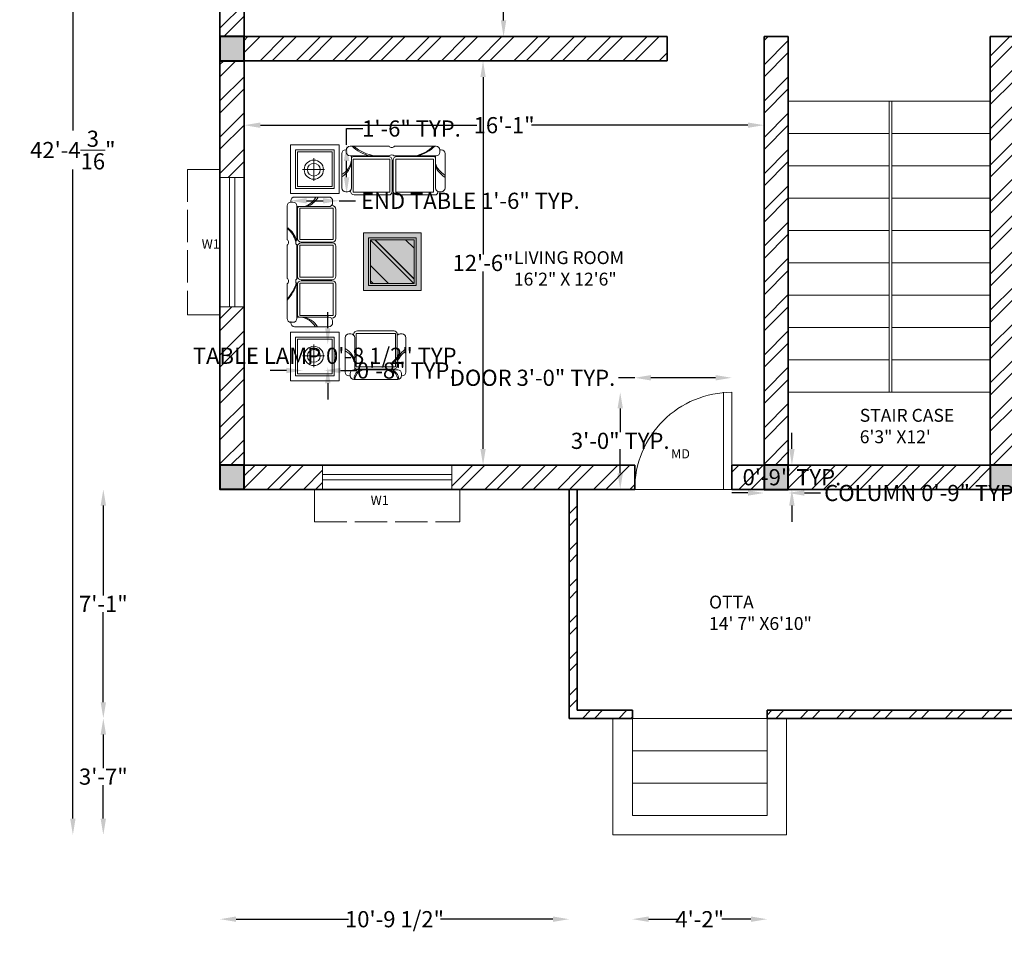
# Model space of a CAD drawing. Units: inches. Extents: x 3614 to 4242, y 2406 to 3033.
# Tile 1 of 10: x 3614 to 3980, y 2406 to 2749. Entities that reach past the tile are written whole.
import ezdxf

# ---------------------------------------------------------------- set-up
doc = ezdxf.new("R2010")
doc.units = ezdxf.units.IN
doc.linetypes.add('ACAD_ISO02W100', pattern=[15, 12, -3])
for name, color, linetype, lineweight in [('A-ANNO-DIMS', 2, 'Continuous', 18), ('A-ANNO-TEXT', 7, 'Continuous', 18), ('A-AREA-IDEN', 7, 'Continuous', 25), ('A-COLS', 7, 'Continuous', 40), ('A-COLS-PATT', 252, 'Continuous', 18), ('A-DOOR', 3, 'Continuous', 18), ('A-FLOR-STRS', 7, 'Continuous', 18), ('A-FURN', 8, 'Continuous', 18), ('A-FURN-PATT', 252, 'Continuous', 13), ('A-GLAZ', 4, 'Continuous', 18), ('A-GLAZ-OVHD', 8, 'ACAD_ISO02W100', 13), ('A-WALL', 7, 'Continuous', 35), ('A-WALL-PATT', 252, 'Continuous', 13)]:
    doc.layers.add(name, color=color, linetype=linetype, lineweight=lineweight)
doc.styles.get("Standard").update_dxf_attribs({"font": 'arial.ttf'})
doc.dimstyles.get("Standard").update_dxf_attribs({"dimtxt": 6, "dimasz": 6, "dimexe": 0.18, "dimexo": 0.0625, "dimgap": 0.09, "dimtad": 0, "dimtih": 1, "dimtoh": 1, "dimdec": 4, "dimzin": 0, "dimdsep": 46, "dimlunit": 4, "dimtxsty": 'Standard', "dimcen": 0.09, "dimse1": 1, "dimse2": 1, "dimadec": 0, "dimazin": 0, "dimtfac": 1, "dimtdec": 4, "dimtofl": 0, "dimtmove": 0, "dimatfit": 3, "dimfxl": 1, "dimtolj": 1, "dimtzin": 0, "dimarcsym": 0})

# ---------------------------------------------------------------- blocks, each defined once
blk = doc.blocks.new('*D15')
at = {"layer": 'A-ANNO-DIMS', "color": 0, "lineweight": -2, "transparency": 16777216}
for p, q in [((3793.63, 2939.34), (3793.63, 2846.99)), ((3793.63, 2748.34), (3793.63, 2840.69))]:
    blk.add_line(p, q, dxfattribs=at)
at = {"layer": 'A-ANNO-DIMS', "color": 0, "transparency": 16777216}
for points in [[(3792.63, 2939.34), (3794.63, 2939.34), (3793.63, 2945.34)], [(3792.63, 2748.34), (3794.63, 2748.34), (3793.63, 2742.34)]]:
    blk.add_solid(points, dxfattribs=at)
at = {"layer": 'Defpoints', "color": 0, "transparency": 16777216}
for p in [(3799.84, 2945.34), (3793.63, 2742.34), (3799.84, 2742.34)]:
    blk.add_point(p, dxfattribs=at)
at = {"layer": 'A-ANNO-DIMS', "color": 0, "transparency": 16777216, "insert": (3793.63, 2843.84), "char_height": 6, "attachment_point": 5}
blk.add_mtext('\\A1;16\'-11"', dxfattribs=at)
blk = doc.blocks.new('*D17')
at = {"layer": 'A-ANNO-DIMS', "color": 0, "lineweight": -2, "transparency": 16777216}
for p, q in [((3786.02, 2727.34), (3786.02, 2661.49)), ((3786.02, 2589.34), (3786.02, 2655.19))]:
    blk.add_line(p, q, dxfattribs=at)
at = {"layer": 'A-ANNO-DIMS', "color": 0, "transparency": 16777216}
for points in [[(3785.02, 2727.34), (3787.02, 2727.34), (3786.02, 2733.34)], [(3785.02, 2589.34), (3787.02, 2589.34), (3786.02, 2583.34)]]:
    blk.add_solid(points, dxfattribs=at)
at = {"layer": 'Defpoints', "color": 0, "transparency": 16777216}
for p in [(3831.84, 2733.34), (3786.02, 2583.34), (3830.34, 2583.34)]:
    blk.add_point(p, dxfattribs=at)
at = {"layer": 'A-ANNO-DIMS', "color": 0, "transparency": 16777216, "insert": (3786.02, 2658.34), "char_height": 6, "attachment_point": 5}
blk.add_mtext('\\A1;12\'-6"', dxfattribs=at)
blk = doc.blocks.new('*D18')
at = {"layer": 'A-ANNO-DIMS', "color": 0, "lineweight": -2, "transparency": 16777216}
for p, q in [((3703.34, 2709.47), (3783.72, 2709.47)), ((3884.34, 2709.47), (3803.95, 2709.47))]:
    blk.add_line(p, q, dxfattribs=at)
at = {"layer": 'A-ANNO-DIMS', "color": 0, "transparency": 16777216}
for points in [[(3703.34, 2710.47), (3703.34, 2708.47), (3697.34, 2709.47)], [(3884.34, 2710.47), (3884.34, 2708.47), (3890.34, 2709.47)]]:
    blk.add_solid(points, dxfattribs=at)
at = {"layer": 'Defpoints', "color": 0, "transparency": 16777216}
for p in [(3890.34, 2709.47), (3697.34, 2600.55), (3890.34, 2600.55)]:
    blk.add_point(p, dxfattribs=at)
at = {"layer": 'A-ANNO-DIMS', "color": 0, "transparency": 16777216, "insert": (3793.84, 2709.47), "char_height": 6, "attachment_point": 5}
blk.add_mtext('\\A1;16\'-1"', dxfattribs=at)
blk = doc.blocks.new('*D26')
at = {"layer": 'A-ANNO-DIMS', "color": 0, "lineweight": -2, "transparency": 16777216}
for p, q in [((3633.72, 2948.34), (3633.72, 2707.46)), ((3633.72, 2452.14), (3633.72, 2693.02))]:
    blk.add_line(p, q, dxfattribs=at)
at = {"layer": 'A-ANNO-DIMS', "color": 0, "transparency": 16777216}
for points in [[(3632.72, 2948.34), (3634.72, 2948.34), (3633.72, 2954.34)], [(3632.72, 2452.14), (3634.72, 2452.14), (3633.72, 2446.14)]]:
    blk.add_solid(points, dxfattribs=at)
at = {"layer": 'Defpoints', "color": 0, "transparency": 16777216}
for p in [(3688.34, 2954.34), (3633.72, 2446.14), (3688.34, 2446.14)]:
    blk.add_point(p, dxfattribs=at)
at = {"layer": 'A-ANNO-DIMS', "color": 0, "transparency": 16777216, "insert": (3633.72, 2700.24), "char_height": 6, "attachment_point": 5}
blk.add_mtext('\\A1;42\'-4{\\H1x;\\S3/16;}"', dxfattribs=at)
blk = doc.blocks.new('WINDOW-W1-48IN')
for p, q in [((48, 9), (0, 9)), ((0, 9), (0, 0)), ((48, 0), (48, 9)), ((0, 5.5), (48, 5.5)), ((0, 3.5), (48, 3.5)), ((0, 0), (48, 0))]:
    blk.add_line(p, q)
blk = doc.blocks.new('SHADE-W1')
for p, q in [((0, 0), (0, 12)), ((0, 12), (51, 12)), ((51, 12), (54, 12)), ((54, 12), (54, 0)), ((3, 0), (0, 0))]:
    blk.add_line(p, q)
blk = doc.blocks.new('COLUMN-9X9')
blk.add_lwpolyline([(9, 9), (0, 9), (0, 0), (9, 0)], close=True)
blk = doc.blocks.new('DOOR-SWING-36IN')
for p, q in [((0, 36), (0, 0)), ((0, 0), (0, 36)), ((3, 0), (3, 36))]:
    blk.add_line(p, q)
blk.add_arc((0, 36), 36, 270, 0)
blk = doc.blocks.new('TABLE-END-SQUARE')
for p, q in [((18.1, 18.1), (0, 18.1)), ((0, 18.1), (0, 0)), ((16.2, 16.2), (1.91, 16.2)), ((1.91, 16.2), (1.91, 1.91)), ((15.48, 15.48), (2.62, 15.48)), ((2.62, 15.48), (2.62, 2.62)), ((15.48, 2.62), (15.48, 15.48)), ((16.2, 1.91), (16.2, 16.2)), ((18.1, 0), (18.1, 18.1)), ((0, 0), (18.1, 0)), ((1.91, 1.91), (16.2, 1.91)), ((2.62, 2.62), (15.48, 2.62))]:
    blk.add_line(p, q)
blk = doc.blocks.new('LAMP-TABLE-PLAN')
for p, q in [((4.15, 0), (4.15, 8.41)), ((0, 4.15), (8.06, 4.15))]:
    blk.add_line(p, q)
for radius in [3.57, 2.38]:
    blk.add_circle((4.15, 4.15), radius)
blk = doc.blocks.new('*D39')
at = {"layer": 'A-ANNO-DIMS', "color": 0, "lineweight": -2, "transparency": 16777216}
for p, q in [((3884.34, 2572.99), (3878.34, 2572.99)), ((3905.34, 2572.99), (3911.34, 2572.99))]:
    blk.add_line(p, q, dxfattribs=at)
at = {"layer": 'A-ANNO-DIMS', "color": 0, "transparency": 16777216}
for points in [[(3884.34, 2573.99), (3884.34, 2571.99), (3890.34, 2572.99)], [(3905.34, 2573.99), (3905.34, 2571.99), (3899.34, 2572.99)]]:
    blk.add_solid(points, dxfattribs=at)
at = {"layer": 'Defpoints', "color": 0, "transparency": 16777216}
for p in [(3890.34, 2574.34), (3899.34, 2574.34), (3899.34, 2572.99)]:
    blk.add_point(p, dxfattribs=at)
at = {"layer": 'A-ANNO-DIMS', "color": 0, "transparency": 16777216, "insert": (3949, 2572.99), "char_height": 6, "attachment_point": 5}
blk.add_mtext('\\A1;COLUMN 0\'-9" TYP.', dxfattribs=at)
blk = doc.blocks.new('*D40')
at = {"layer": 'A-ANNO-DIMS', "color": 0, "lineweight": -2, "transparency": 16777216}
for p, q in [((3900.69, 2589.34), (3900.69, 2595.34)), ((3900.69, 2568.34), (3900.69, 2562.34))]:
    blk.add_line(p, q, dxfattribs=at)
at = {"layer": 'A-ANNO-DIMS', "color": 0, "transparency": 16777216}
for points in [[(3899.69, 2589.34), (3901.69, 2589.34), (3900.69, 2583.34)], [(3899.69, 2568.34), (3901.69, 2568.34), (3900.69, 2574.34)]]:
    blk.add_solid(points, dxfattribs=at)
at = {"layer": 'Defpoints', "color": 0, "transparency": 16777216}
for p in [(3899.34, 2583.34), (3900.69, 2583.34), (3899.34, 2574.34)]:
    blk.add_point(p, dxfattribs=at)
at = {"layer": 'A-ANNO-DIMS', "color": 0, "transparency": 16777216, "insert": (3900.69, 2578.84), "char_height": 6, "attachment_point": 5}
blk.add_mtext('\\A1;0\'-9" TYP.', dxfattribs=at)
blk = doc.blocks.new('*D49')
at = {"layer": 'A-ANNO-DIMS', "color": 0, "lineweight": -2, "transparency": 16777216}
for p, q in [((3842.34, 2615.74), (3836.34, 2615.74)), ((3872.34, 2615.74), (3848.34, 2615.74))]:
    blk.add_line(p, q, dxfattribs=at)
at = {"layer": 'A-ANNO-DIMS', "color": 0, "transparency": 16777216}
for points in [[(3848.34, 2616.74), (3848.34, 2614.74), (3842.34, 2615.74)], [(3872.34, 2616.74), (3872.34, 2614.74), (3878.34, 2615.74)]]:
    blk.add_solid(points, dxfattribs=at)
at = {"layer": 'Defpoints', "color": 0, "transparency": 16777216}
for p in [(3842.34, 2615.74), (3842.34, 2610.34), (3878.34, 2610.34)]:
    blk.add_point(p, dxfattribs=at)
at = {"layer": 'A-ANNO-DIMS', "color": 0, "transparency": 16777216, "insert": (3804.37, 2615.74), "char_height": 6, "attachment_point": 5}
blk.add_mtext('\\A1;DOOR 3\'-0" TYP.', dxfattribs=at)
blk = doc.blocks.new('*D50')
at = {"layer": 'A-ANNO-DIMS', "color": 0, "lineweight": -2, "transparency": 16777216}
for p, q in [((3836.94, 2604.34), (3836.94, 2595.5)), ((3836.94, 2580.34), (3836.94, 2589.19))]:
    blk.add_line(p, q, dxfattribs=at)
at = {"layer": 'A-ANNO-DIMS', "color": 0, "transparency": 16777216}
for points in [[(3835.94, 2604.34), (3837.94, 2604.34), (3836.94, 2610.34)], [(3835.94, 2580.34), (3837.94, 2580.34), (3836.94, 2574.34)]]:
    blk.add_solid(points, dxfattribs=at)
at = {"layer": 'Defpoints', "color": 0, "transparency": 16777216}
for p in [(3842.34, 2610.34), (3836.94, 2574.34), (3842.34, 2574.34)]:
    blk.add_point(p, dxfattribs=at)
at = {"layer": 'A-ANNO-DIMS', "color": 0, "transparency": 16777216, "insert": (3836.94, 2592.34), "char_height": 6, "attachment_point": 5}
blk.add_mtext('\\A1;3\'-0" TYP.', dxfattribs=at)
blk = doc.blocks.new('*D59')
at = {"layer": 'A-ANNO-DIMS', "color": 0, "lineweight": -2, "transparency": 16777216}
for p, q in [((3720.53, 2681.41), (3726.63, 2681.41)), ((3732.63, 2681.41), (3738.63, 2681.41))]:
    blk.add_line(p, q, dxfattribs=at)
at = {"layer": 'A-ANNO-DIMS', "color": 0, "transparency": 16777216}
for points in [[(3720.53, 2682.41), (3720.53, 2680.41), (3714.53, 2681.41)], [(3726.63, 2682.41), (3726.63, 2680.41), (3732.63, 2681.41)]]:
    blk.add_solid(points, dxfattribs=at)
at = {"layer": 'Defpoints', "color": 0, "transparency": 16777216}
for p in [(3714.53, 2684.13), (3732.63, 2684.13), (3732.63, 2681.41)]:
    blk.add_point(p, dxfattribs=at)
at = {"layer": 'A-ANNO-DIMS', "color": 0, "transparency": 16777216, "insert": (3781.31, 2681.41), "char_height": 6, "attachment_point": 5}
blk.add_mtext('\\A1;END TABLE 1\'-6" TYP.', dxfattribs=at)
blk = doc.blocks.new('*D60')
at = {"layer": 'A-ANNO-DIMS', "color": 0, "lineweight": -2, "transparency": 16777216}
for p, q in [((3735.35, 2702.23), (3735.35, 2708.23)), ((3735.35, 2708.23), (3741.35, 2708.23)), ((3735.35, 2690.13), (3735.35, 2696.23))]:
    blk.add_line(p, q, dxfattribs=at)
at = {"layer": 'A-ANNO-DIMS', "color": 0, "transparency": 16777216}
for points in [[(3734.35, 2696.23), (3736.35, 2696.23), (3735.35, 2702.23)], [(3734.35, 2690.13), (3736.35, 2690.13), (3735.35, 2684.13)]]:
    blk.add_solid(points, dxfattribs=at)
at = {"layer": 'Defpoints', "color": 0, "transparency": 16777216}
for p in [(3732.63, 2702.23), (3735.35, 2702.23), (3732.63, 2684.13)]:
    blk.add_point(p, dxfattribs=at)
at = {"layer": 'A-ANNO-DIMS', "color": 0, "transparency": 16777216, "insert": (3759.44, 2708.23), "char_height": 6, "attachment_point": 5}
blk.add_mtext('\\A1;1\'-6" TYP.', dxfattribs=at)
blk = doc.blocks.new('*D61')
at = {"layer": 'A-ANNO-DIMS', "color": 0, "lineweight": -2, "transparency": 16777216}
for p, q in [((3728.37, 2634.11), (3728.37, 2640.11)), ((3728.37, 2613.7), (3728.37, 2607.7))]:
    blk.add_line(p, q, dxfattribs=at)
at = {"layer": 'A-ANNO-DIMS', "color": 0, "transparency": 16777216}
for points in [[(3727.37, 2634.11), (3729.37, 2634.11), (3728.37, 2628.11)], [(3727.37, 2613.7), (3729.37, 2613.7), (3728.37, 2619.7)]]:
    blk.add_solid(points, dxfattribs=at)
at = {"layer": 'Defpoints', "color": 0, "transparency": 16777216}
for p in [(3727.11, 2628.11), (3728.37, 2628.11), (3727.11, 2619.7)]:
    blk.add_point(p, dxfattribs=at)
at = {"layer": 'A-ANNO-DIMS', "color": 0, "transparency": 16777216, "insert": (3728.37, 2623.9), "char_height": 6, "attachment_point": 5}
blk.add_mtext('\\A1;TABLE LAMP 0\'-8 1/2" TYP.', dxfattribs=at)
blk = doc.blocks.new('*D62')
at = {"layer": 'A-ANNO-DIMS', "color": 0, "lineweight": -2, "transparency": 16777216}
for p, q in [((3713.04, 2618.44), (3707.04, 2618.44)), ((3733.11, 2618.44), (3739.11, 2618.44))]:
    blk.add_line(p, q, dxfattribs=at)
at = {"layer": 'A-ANNO-DIMS', "color": 0, "transparency": 16777216}
for points in [[(3713.04, 2619.44), (3713.04, 2617.44), (3719.04, 2618.44)], [(3733.11, 2619.44), (3733.11, 2617.44), (3727.11, 2618.44)]]:
    blk.add_solid(points, dxfattribs=at)
at = {"layer": 'Defpoints', "color": 0, "transparency": 16777216}
for p in [(3719.04, 2619.7), (3727.11, 2619.7), (3727.11, 2618.44)]:
    blk.add_point(p, dxfattribs=at)
at = {"layer": 'A-ANNO-DIMS', "color": 0, "transparency": 16777216, "insert": (3757.48, 2618.44), "char_height": 6, "attachment_point": 5}
blk.add_mtext('\\A1;0\'-8" TYP.', dxfattribs=at)
blk = doc.blocks.new('*D67')
at = {"layer": 'A-ANNO-DIMS', "color": 0, "lineweight": -2, "transparency": 16777216}
for p, q in [((3694.34, 2414.84), (3736.04, 2414.84)), ((3811.95, 2414.84), (3770.25, 2414.84))]:
    blk.add_line(p, q, dxfattribs=at)
at = {"layer": 'A-ANNO-DIMS', "color": 0, "transparency": 16777216}
for points in [[(3694.34, 2415.84), (3694.34, 2413.84), (3688.34, 2414.84)], [(3811.95, 2415.84), (3811.95, 2413.84), (3817.95, 2414.84)]]:
    blk.add_solid(points, dxfattribs=at)
at = {"layer": 'Defpoints', "color": 0, "transparency": 16777216}
for p in [(3688.34, 2574.34), (3817.95, 2574.34), (3817.95, 2414.84)]:
    blk.add_point(p, dxfattribs=at)
at = {"layer": 'A-ANNO-DIMS', "color": 0, "transparency": 16777216, "insert": (3753.14, 2414.84), "char_height": 6, "attachment_point": 5}
blk.add_mtext('\\A1;10\'-9 1/2"', dxfattribs=at)
blk = doc.blocks.new('*D68')
at = {"layer": 'A-ANNO-DIMS', "color": 0, "lineweight": -2, "transparency": 16777216}
for p, q in [((3645.04, 2568.34), (3645.04, 2534.94)), ((3645.04, 2495.34), (3645.04, 2528.74))]:
    blk.add_line(p, q, dxfattribs=at)
at = {"layer": 'A-ANNO-DIMS', "color": 0, "transparency": 16777216}
for points in [[(3644.04, 2568.34), (3646.04, 2568.34), (3645.04, 2574.34)], [(3644.04, 2495.34), (3646.04, 2495.34), (3645.04, 2489.34)]]:
    blk.add_solid(points, dxfattribs=at)
at = {"layer": 'Defpoints', "color": 0, "transparency": 16777216}
for p in [(3645.04, 2574.34), (3817.95, 2574.34), (3817.95, 2489.34)]:
    blk.add_point(p, dxfattribs=at)
at = {"layer": 'A-ANNO-DIMS', "color": 0, "transparency": 16777216, "insert": (3645.04, 2531.84), "char_height": 6, "attachment_point": 5}
blk.add_mtext('\\A1;7\'-1"', dxfattribs=at)
blk = doc.blocks.new('*D69')
at = {"layer": 'A-ANNO-DIMS', "color": 0, "lineweight": -2, "transparency": 16777216}
for p, q in [((3847.46, 2414.84), (3858.28, 2414.84)), ((3885.48, 2414.84), (3874.65, 2414.84))]:
    blk.add_line(p, q, dxfattribs=at)
at = {"layer": 'A-ANNO-DIMS', "color": 0, "transparency": 16777216}
for points in [[(3847.46, 2415.84), (3847.46, 2413.84), (3841.46, 2414.84)], [(3885.48, 2415.84), (3885.48, 2413.84), (3891.48, 2414.84)]]:
    blk.add_solid(points, dxfattribs=at)
at = {"layer": 'Defpoints', "color": 0, "transparency": 16777216}
for p in [(3841.46, 2453.34), (3891.48, 2453.34), (3891.48, 2414.84)]:
    blk.add_point(p, dxfattribs=at)
at = {"layer": 'A-ANNO-DIMS', "color": 0, "transparency": 16777216, "insert": (3866.47, 2414.84), "char_height": 6, "attachment_point": 5}
blk.add_mtext('\\A1;4\'-2"', dxfattribs=at)
blk = doc.blocks.new('*D70')
at = {"layer": 'A-ANNO-DIMS', "color": 0, "lineweight": -2, "transparency": 16777216}
for p, q in [((3645.04, 2483.34), (3645.04, 2470.9)), ((3645.04, 2452.14), (3645.04, 2464.59))]:
    blk.add_line(p, q, dxfattribs=at)
at = {"layer": 'A-ANNO-DIMS', "color": 0, "transparency": 16777216}
for points in [[(3644.04, 2483.34), (3646.04, 2483.34), (3645.04, 2489.34)], [(3644.04, 2452.14), (3646.04, 2452.14), (3645.04, 2446.14)]]:
    blk.add_solid(points, dxfattribs=at)
at = {"layer": 'Defpoints', "color": 0, "transparency": 16777216}
for p in [(3645.04, 2489.34), (3834.26, 2489.34), (3834.26, 2446.14)]:
    blk.add_point(p, dxfattribs=at)
at = {"layer": 'A-ANNO-DIMS', "color": 0, "transparency": 16777216, "insert": (3645.04, 2467.74), "char_height": 6, "attachment_point": 5}
blk.add_mtext('\\A1;3\'-7"', dxfattribs=at)

msp = doc.modelspace()

# ---------------------------------------------------------------- hatches: boundary and pattern name
at = {"layer": 'A-COLS-PATT'}
h = msp.add_hatch(color=256, dxfattribs=at)
h.dxf.hatch_style = 1
h.paths.add_polyline_path([(3697.336, 2954.34049), (3688.336, 2954.34049), (3688.336, 2945.34049), (3697.336, 2945.34049)])
h.paths.add_polyline_path([(3818.336, 2954.34049), (3809.336, 2954.34049), (3809.336, 2945.34049), (3818.336, 2945.34049)])
h.paths.add_polyline_path([(3818.336, 2787.28572), (3809.336, 2787.28572), (3809.336, 2778.34049), (3818.336, 2778.34049)])
h.paths.add_polyline_path([(3697.336, 2742.34049), (3688.336, 2742.34049), (3688.336, 2733.34049), (3697.336, 2733.34049)])
h.paths.add_polyline_path([(3697.336, 2583.37355), (3688.336, 2583.37355), (3688.336, 2574.37355), (3697.336, 2574.37355)])
h.paths.add_polyline_path([(3899.336, 2583.34049), (3890.336, 2583.34049), (3890.336, 2574.34049), (3899.336, 2574.34049)])
h.paths.add_polyline_path([(3983.336, 2583.34049), (3974.336, 2583.34049), (3974.336, 2574.34049), (3983.336, 2574.34049)])
h.paths.add_polyline_path([(4153.336, 2583.34049), (4144.336, 2583.34049), (4144.336, 2574.34049), (4153.336, 2574.34049)])
h.paths.add_polyline_path([(4153.336, 2742.34049), (4144.336, 2742.34049), (4144.336, 2733.34049), (4153.336, 2733.34049)])
h.paths.add_polyline_path([(4153.336, 2795.34049), (4144.336, 2795.34049), (4144.336, 2786.34049), (4153.336, 2786.34049)])
h.paths.add_polyline_path([(3983.336, 2795.31105), (3974.336, 2795.31105), (3974.336, 2786.34049), (3983.336, 2786.34049)])
h.paths.add_polyline_path([(4153.336, 2954.34049), (4144.36882, 2954.34049), (4144.36882, 2945.34049), (4153.336, 2945.34049)])
h.paths.add_polyline_path([(3982.96188, 2954.34049), (3973.96188, 2954.34049), (3973.96188, 2945.34049), (3982.96188, 2945.34049)])
at = {"layer": 'A-FURN-PATT'}
h = msp.add_hatch(dxfattribs=at)
h.set_pattern_fill('CROSS', color=256, scale=0.833737, angle=135, style=0)
h.set_pattern_definition([(135, (1285.79775, 1101.19767), (-0.294770579, 0), [0.104217138, -0.312651413]), (225, (1285.79775, 1101.27136), (0, -0.294770579), [0.104217138, -0.312651413])])
h.paths.add_polyline_path([(3763.05675, 2669.55465), (3741.6178, 2669.55465), (3741.6178, 2648.11569), (3763.05675, 2648.11569)])
h = msp.add_hatch(dxfattribs=at)
h.set_pattern_fill('AR-RROOF', color=256, scale=11.91053, angle=135, style=0)
h.set_pattern_definition([(135, (1285.798, 1101.198), (-26.950453, 10.10642), [178.65795, -23.82106, 59.55265, -11.91053]), (135, (1270.385, 1108.188), (-2.779265, -19.6233), [35.7316, -3.93047, 71.46318, -8.9329]), (135, (1274.428, 1098.25), (-49.437237, 38.151735), [95.28424, -16.67474, 47.64212, -11.91053])])
h.paths.add_polyline_path([(3760.43644, 2666.93433), (3744.23811, 2666.93433), (3744.23811, 2650.73601), (3760.43644, 2650.73601)])
at = {"layer": 'A-WALL-PATT'}
h = msp.add_hatch(dxfattribs=at)
h.set_pattern_fill('ANSI32', color=256)
h.paths.add_polyline_path([(4153.336, 2945.34049), (4144.336, 2945.34049), (4144.336, 2902.95478), (4153.336, 2902.95478)])
h.paths.add_polyline_path([(4144.36882, 2954.34049), (4089.01458, 2954.34049), (4089.01458, 2945.34049), (4144.36882, 2945.34049)])
h.paths.add_polyline_path([(3818.336, 2945.34049), (3809.336, 2945.34049), (3809.336, 2787.28572), (3818.336, 2787.28572)])
h.paths.add_polyline_path([(3697.336, 2846.73438), (3688.336, 2846.73438), (3688.336, 2742.34049), (3697.336, 2742.34049)])
h.paths.add_polyline_path([(3854.336, 2742.34049), (3853.36389, 2742.34049), (3818.336, 2742.34049), (3809.336, 2742.34049), (3697.336, 2742.34049), (3697.336, 2733.34049), (3809.336, 2733.34049), (3854.336, 2733.34049)])
h.paths.add_polyline_path([(3697.336, 2733.34049), (3688.336, 2733.34049), (3688.336, 2690.05693), (3697.336, 2690.05693)])
h.paths.add_polyline_path([(3697.336, 2642.05693), (3688.336, 2642.05693), (3688.336, 2583.37355), (3697.336, 2583.37355)])
h.paths.add_polyline_path([(3726.39802, 2583.34049), (3697.336, 2583.34049), (3697.336, 2574.34049), (3726.39802, 2574.34049)])
h.paths.add_polyline_path([(3842.336, 2583.34049), (3818.336, 2583.34049), (3809.336, 2583.34049), (3774.39802, 2583.34049), (3774.39802, 2574.34049), (3809.336, 2574.34049), (3842.336, 2574.34049)])
h.paths.add_polyline_path([(3890.336, 2583.34049), (3878.336, 2583.34049), (3878.336, 2574.34049), (3890.336, 2574.34049)])
h = msp.add_hatch(dxfattribs=at)
h.set_pattern_fill('ANSI32', color=256)
h.paths.add_polyline_path([(3899.336, 2733.34049), (3899.336, 2742.34049), (3890.336, 2742.34049), (3890.336, 2583.34049), (3899.336, 2583.34049)])
h.paths.add_polyline_path([(3983.336, 2733.34049), (3995.336, 2733.34049), (3995.336, 2742.34049), (3983.336, 2742.34049), (3974.336, 2742.34049), (3974.336, 2583.34049), (3983.336, 2583.34049)])
h.paths.add_polyline_path([(3974.336, 2583.34049), (3899.336, 2583.34049), (3899.336, 2574.34049), (3974.336, 2574.34049)])
h.paths.add_polyline_path([(4045.73114, 2583.34049), (3983.336, 2583.34049), (3983.336, 2574.34049), (4045.73114, 2574.34049)])
h.paths.add_polyline_path([(4144.336, 2583.34049), (4093.73114, 2583.34049), (4093.73114, 2574.34049), (4144.336, 2574.34049)])
h.paths.add_polyline_path([(4153.336, 2639.00845), (4144.336, 2639.00845), (4144.336, 2583.34049), (4153.336, 2583.34049)])
h.paths.add_polyline_path([(4153.336, 2733.34049), (4144.336, 2733.34049), (4144.336, 2687.00845), (4153.336, 2687.00845)])
h.paths.add_polyline_path([(4144.336, 2742.34049), (4096.76112, 2742.34049, -0.076320834), (4098.14294, 2733.34049), (4144.336, 2733.34049)])
h.paths.add_polyline_path([(4068.14294, 2742.34049), (4056.14294, 2742.34049), (4031.336, 2742.34049, -0.063254224), (4030.19285, 2733.34049), (4068.14294, 2733.34049)])
h.paths.add_polyline_path([(4144.336, 2795.34049), (4042.336, 2795.34049), (4042.336, 2786.34049), (4144.336, 2786.34049)])
h.paths.add_polyline_path([(4153.336, 2854.95478), (4144.336, 2854.95478), (4144.336, 2795.34049), (4153.336, 2795.34049)])
h = msp.add_hatch(dxfattribs=at)
h.set_pattern_fill('ANSI32', color=256)
h.paths.add_polyline_path([(3820.94922, 2574.34049), (3817.94922, 2574.34049), (3817.94922, 2489.34049), (3841.45991, 2489.34049), (3841.45991, 2492.34049), (3820.94922, 2492.34049)])
h = msp.add_hatch(dxfattribs=at)
h.set_pattern_fill('ANSI32', color=256)
h.paths.add_polyline_path([(3983.336, 2492.34049), (3891.47836, 2492.34049), (3891.47836, 2489.34049), (3983.336, 2489.34049)])
h.paths.add_polyline_path([(3986.336, 2574.34049), (3983.336, 2574.34049), (3983.336, 2492.34049), (3983.336, 2489.34049), (3986.336, 2489.34049)])

# ---------------------------------------------------------------- linework, layer by layer
at = {"layer": 'A-DOOR'}
msp.add_line((3878.336, 2574.34049), (3842.336, 2574.34049), dxfattribs=at)
at = {"layer": 'A-FLOR-STRS'}
for p, q in [((3899.336, 2718.34049), (3974.336, 2718.34049)), ((3936.836, 2610.34049), (3936.836, 2718.34049)), ((3937.836, 2610.34049), (3937.836, 2718.34049)), ((3899.336, 2706.34049), (3936.836, 2706.34049)), ((3937.836, 2706.34049), (3974.336, 2706.34049)), ((3899.336, 2694.34049), (3936.836, 2694.34049)), ((3937.836, 2694.34049), (3974.336, 2694.34049)), ((3899.336, 2682.34049), (3936.836, 2682.34049)), ((3937.836, 2682.34049), (3974.336, 2682.34049)), ((3899.336, 2670.34049), (3936.836, 2670.34049)), ((3937.836, 2670.34049), (3974.336, 2670.34049)), ((3899.336, 2658.34049), (3936.836, 2658.34049)), ((3937.836, 2658.34049), (3974.336, 2658.34049)), ((3899.336, 2646.34049), (3936.836, 2646.34049)), ((3937.836, 2646.34049), (3974.336, 2646.34049)), ((3899.336, 2634.34049), (3936.836, 2634.34049)), ((3937.836, 2634.34049), (3974.336, 2634.34049)), ((3974.336, 2634.34049), (3974.33588, 2634.34049)), ((3899.336, 2622.34049), (3936.836, 2622.34049)), ((3937.836, 2622.34049), (3974.336, 2622.34049)), ((3899.336, 2610.34049), (3974.336, 2610.34049)), ((3834.25991, 2489.34049), (3834.25991, 2453.34049)), ((3841.45991, 2489.34049), (3841.45991, 2453.34049)), ((3841.45991, 2489.34049), (3891.47836, 2489.34049)), ((3891.47836, 2453.34049), (3891.47836, 2489.34049)), ((3898.67836, 2453.34049), (3898.67836, 2489.34049)), ((3841.45991, 2477.34049), (3891.47836, 2477.34049)), ((3841.45991, 2465.34049), (3891.47836, 2465.34049)), ((3834.25991, 2453.34049), (3834.25991, 2446.14049)), ((3841.45991, 2453.34049), (3891.47836, 2453.34049)), ((3898.67836, 2446.14049), (3898.67836, 2453.34049)), ((3834.25991, 2446.14049), (3898.67836, 2446.14049))]:
    msp.add_line(p, q, dxfattribs=at)
at = {"layer": 'A-FURN'}
for p, q in [((3751.13641, 2701.64891), (3736.64593, 2701.64891)), ((3768.46047, 2701.64891), (3753.14251, 2701.64891)), ((3733.60133, 2686.19861), (3733.60133, 2698.91193)), ((3735.48679, 2700.34119), (3735.0306, 2700.34119)), ((3735.21666, 2700.21964), (3735.21666, 2699.50501)), ((3751.22261, 2698.07575), (3736.64593, 2698.07575)), ((3737.17449, 2686.19861), (3737.17449, 2698.17708)), ((3750.84644, 2697.88006), (3738.21952, 2697.88006)), ((3768.54667, 2698.07575), (3753.05631, 2698.07575)), ((3767.62122, 2697.88006), (3754.03089, 2697.88006)), ((3768.34346, 2686.19861), (3768.34346, 2698.0934)), ((3769.99665, 2700.21964), (3769.99665, 2699.50501)), ((3770.03117, 2700.34119), (3770.48736, 2700.34119)), ((3771.91662, 2686.19861), (3771.91662, 2698.91193)), ((3737.77099, 2684.60545), (3737.77099, 2696.91366)), ((3737.77099, 2696.91366), (3751.38367, 2696.91366)), ((3751.38367, 2696.91366), (3751.38367, 2684.60545)), ((3752.27571, 2696.4508), (3752.27571, 2684.77848)), ((3752.60163, 2696.4508), (3752.60163, 2685.01669)), ((3753.58237, 2684.60545), (3753.58237, 2696.91366)), ((3753.58237, 2696.91366), (3767.645, 2696.91366)), ((3767.645, 2696.91366), (3767.645, 2684.60545)), ((3735.74523, 2684.76935), (3735.0306, 2684.76935)), ((3736.79025, 2685.24035), (3736.79025, 2685.01669)), ((3751.38367, 2684.60545), (3737.77099, 2684.60545)), ((3751.08465, 2683.58742), (3738.21952, 2683.58742)), ((3767.645, 2684.60545), (3753.58237, 2684.60545)), ((3768.09975, 2683.58742), (3754.03089, 2683.58742)), ((3769.2908, 2684.85305), (3769.2908, 2684.77848)), ((3769.77273, 2684.76935), (3770.48736, 2684.76935)), ((3714.6077, 2680.93085), (3714.6077, 2681.38705)), ((3714.72925, 2680.94456), (3715.44389, 2680.94456)), ((3728.75028, 2682.81631), (3716.03697, 2682.81631)), ((3729.72533, 2679.62739), (3729.93221, 2679.62739)), ((3730.17955, 2680.67241), (3730.17955, 2681.38705)), ((3713.29999, 2679.51529), (3713.29999, 2666.96796)), ((3728.75028, 2679.24315), (3716.77182, 2679.24315)), ((3716.87315, 2679.51529), (3716.87315, 2666.88176)), ((3717.06884, 2667.5465), (3717.06884, 2678.19813)), ((3730.34345, 2678.64666), (3718.03524, 2678.64666)), ((3718.03524, 2678.64666), (3718.03524, 2667.00927)), ((3730.34345, 2667.00927), (3730.34345, 2678.64666)), ((3731.36147, 2667.30829), (3731.36147, 2678.19813)), ((3763.05675, 2669.55465), (3741.6178, 2669.55465)), ((3741.6178, 2669.55465), (3741.6178, 2648.11569)), ((3763.05675, 2648.11569), (3763.05675, 2669.55465)), ((3713.29999, 2664.96186), (3713.29999, 2652.59543)), ((3716.87315, 2665.04806), (3716.87315, 2652.50923)), ((3718.03524, 2667.00927), (3730.34345, 2667.00927)), ((3718.4981, 2666.11723), (3730.17042, 2666.11723)), ((3718.4981, 2665.79219), (3730.17042, 2665.79219)), ((3761.15107, 2667.64896), (3743.52348, 2667.64896)), ((3743.52348, 2667.64896), (3743.52348, 2650.02138)), ((3760.43644, 2666.93433), (3744.23811, 2666.93433)), ((3744.23811, 2666.93433), (3744.23811, 2650.73601)), ((3760.43644, 2650.73601), (3760.43644, 2666.93433)), ((3761.15107, 2650.02138), (3761.15107, 2667.64896)), ((3717.06884, 2664.36293), (3717.06884, 2653.48381)), ((3718.03524, 2664.90015), (3730.34345, 2664.90015)), ((3718.03524, 2653.03528), (3718.03524, 2664.90015)), ((3730.34345, 2664.90015), (3730.34345, 2653.03528)), ((3731.36147, 2664.60114), (3731.36147, 2653.48381)), ((3713.29999, 2650.58933), (3713.29999, 2637.74719)), ((3716.87315, 2650.67553), (3716.87315, 2637.74719)), ((3730.34345, 2653.03528), (3718.03524, 2653.03528)), ((3718.03524, 2650.83658), (3730.34345, 2650.83658)), ((3718.03524, 2638.87225), (3718.03524, 2650.83658)), ((3718.4981, 2652.05455), (3729.93221, 2652.05455)), ((3718.4981, 2651.72862), (3730.17042, 2651.72862)), ((3730.34345, 2650.83658), (3730.34345, 2638.87225)), ((3731.36147, 2650.53757), (3731.36147, 2639.32078)), ((3744.23811, 2650.73601), (3760.43644, 2650.73601)), ((3717.06884, 2650.29936), (3717.06884, 2639.32078)), ((3741.6178, 2648.11569), (3763.05675, 2648.11569)), ((3743.52348, 2650.02138), (3761.15107, 2650.02138)), ((3714.6077, 2636.58806), (3714.6077, 2636.13186)), ((3714.72925, 2636.31793), (3715.44389, 2636.31793)), ((3728.75028, 2638.27576), (3716.77182, 2638.27576)), ((3730.34345, 2638.87225), (3718.03524, 2638.87225)), ((3729.70855, 2637.89152), (3729.93221, 2637.89152)), ((3730.17955, 2636.8465), (3730.17955, 2636.13186)), ((3728.75028, 2634.7026), (3716.03697, 2634.7026)), ((3753.48061, 2632.16529), (3738.9587, 2632.16529)), ((3738.9587, 2632.16529), (3738.9587, 2619.85709)), ((3752.9893, 2633.18332), (3739.40723, 2633.18332)), ((3753.48061, 2619.85709), (3753.48061, 2632.16529)), ((3734.78905, 2630.57213), (3734.78905, 2617.85881)), ((3736.93295, 2632.00139), (3736.21831, 2632.00139)), ((3737.97797, 2631.54718), (3737.97797, 2631.75406)), ((3738.36221, 2630.57213), (3738.36221, 2618.59367)), ((3754.18035, 2620.31995), (3754.18035, 2631.99227)), ((3755.24733, 2632.00139), (3755.96196, 2632.00139)), ((3757.39122, 2630.57213), (3757.39122, 2617.85881)), ((3738.09007, 2618.695), (3754.34663, 2618.695)), ((3738.9587, 2619.85709), (3753.48061, 2619.85709)), ((3752.75109, 2618.89069), (3739.40723, 2618.89069)), ((3736.67451, 2616.42955), (3736.21831, 2616.42955)), ((3736.6608, 2616.5511), (3736.6608, 2617.26573)), ((3738.09007, 2615.12184), (3754.34663, 2615.12184)), ((3755.77589, 2616.5511), (3755.77589, 2617.26573)), ((3755.77589, 2616.42955), (3755.96196, 2616.42955))]:
    msp.add_line(p, q, dxfattribs=at)
for centre, radius, start, end in [((3736.64593, 2700.21964), 1.42926, 90, 180), ((3747.56154, 2712.42936), 14.81213, 226.7033204, 254.9108489), ((3748.39437, 2714.40157), 16.48384, 230.3907627, 262.0602504), ((3752.13946, 2702.3646), 1.23221, 215.50856, 324.49144), ((3758.56588, 2710.62812), 12.7217, 279.35882, 315.4424582), ((3757.95427, 2712.42936), 14.81213, 285.0891511, 313.2966796), ((3768.56738, 2700.21964), 1.42926, 0, 90), ((3735.0306, 2698.91193), 1.42926, 90, 180), ((3736.64593, 2699.50501), 1.42926, 180, 270), ((3738.21952, 2696.4508), 1.42926, 90, 136.9838581), ((3750.84644, 2696.4508), 1.42926, 0, 90), ((3752.13946, 2697.25251), 1.23221, 41.9206973, 138.0793027), ((3754.03089, 2696.4508), 1.42926, 90, 180), ((3767.65376, 2697.06991), 0.81081, 31.7185097, 92.2998875), ((3768.56738, 2699.50501), 1.42926, 270, 0), ((3770.48736, 2698.91193), 1.42926, 0, 90), ((3729.41209, 2697.7734), 7.85392, 302.2352052, 351.9364077), ((3729.41209, 2696.97911), 7.85392, 302.2352052, 351.9364077), ((3775.77734, 2697.7734), 7.85392, 198.8232285, 239.8897989), ((3775.77734, 2696.97911), 7.85392, 198.8232285, 239.8897989), ((3735.0306, 2686.19861), 1.42926, 180, 270), ((3735.74523, 2686.2154), 1.42926, 270, 0), ((3738.21952, 2685.01669), 1.42926, 180, 270), ((3751.08465, 2684.77848), 1.19105, 270, 0), ((3754.03089, 2685.01669), 1.42926, 180, 270), ((3768.09975, 2684.77848), 1.19105, 270, 0), ((3769.77273, 2686.19861), 1.42926, 180, 270), ((3770.48736, 2686.19861), 1.42926, 270, 0), ((3714.72925, 2679.51529), 1.42926, 90, 180), ((3716.03697, 2681.38705), 1.42926, 90, 180), ((3715.44389, 2679.51529), 1.42926, 0, 90), ((3717.1755, 2686.67703), 7.85392, 288.8232284, 329.8897989), ((3717.96979, 2686.67703), 7.85392, 288.8232284, 329.8897989), ((3728.75028, 2681.38705), 1.42926, 0, 90), ((3728.75028, 2680.67241), 1.42926, 270, 0), ((3729.93221, 2678.19813), 1.42926, 0, 90), ((3718.4981, 2678.19813), 1.42926, 133.016142, 180), ((3707.72484, 2664.05606), 9.02945, 13.8700854, 51.2300582), ((3709.22318, 2665.05867), 7.62254, 12.0983755, 55.7660865), ((3712.58429, 2665.96491), 1.23221, 305.50856, 54.49144), ((3717.69639, 2665.96491), 1.23221, 131.9206972, 228.0793028), ((3718.4981, 2667.5465), 1.42926, 180, 270), ((3718.4981, 2664.36293), 1.42926, 90, 180), ((3730.17042, 2667.30829), 1.19105, 270, 0), ((3730.17042, 2664.60114), 1.19105, 0, 90), ((3704.32078, 2654.10089), 12.7217, 314.5575416, 346.4540441), ((3712.58429, 2651.59238), 1.23221, 305.50856, 54.49144), ((3702.51953, 2654.71251), 14.81213, 316.7033206, 344.910849), ((3717.69639, 2651.59238), 1.23221, 131.9206972, 228.0793028), ((3718.4981, 2653.48381), 1.42926, 180, 270), ((3718.4981, 2650.29936), 1.42926, 90, 180), ((3729.93221, 2653.48381), 1.42926, 270, 0), ((3730.17042, 2650.53757), 1.19105, 0, 90), ((3714.72925, 2637.74719), 1.42926, 180, 270), ((3716.03697, 2636.13186), 1.42926, 180, 270), ((3715.44389, 2637.74719), 1.42926, 270, 0), ((3718.4981, 2639.32078), 1.42926, 180, 226.983858), ((3717.1755, 2630.51335), 7.85392, 32.2352053, 81.9364077), ((3717.96979, 2630.51335), 7.85392, 32.2352053, 81.9364077), ((3728.7335, 2636.8465), 1.42926, 0, 90), ((3728.75028, 2636.13186), 1.42926, 270, 0), ((3729.93221, 2639.32078), 1.42926, 270, 0), ((3739.40723, 2631.75406), 1.42926, 90, 180), ((3752.77304, 2631.75406), 1.42926, 0, 90), ((3736.21831, 2630.57213), 1.42926, 90, 180), ((3736.93295, 2630.57213), 1.42926, 0, 90), ((3755.24733, 2630.55535), 1.42926, 90, 138.2900186), ((3755.96196, 2630.57213), 1.42926, 0, 90), ((3730.92833, 2619.79164), 7.85392, 8.0635923, 59.8897989), ((3730.92833, 2618.99735), 7.85392, 8.0635923, 59.8897989), ((3761.58047, 2619.79164), 7.85392, 122.2352052, 160.4278708), ((3761.58047, 2618.99735), 7.85392, 122.2352052, 160.4278708), ((3736.21831, 2617.85881), 1.42926, 180, 270), ((3738.09007, 2617.26573), 1.42926, 90, 180), ((3741.41449, 2615.4856), 3.24527, 103.377287, 182.6905421), ((3739.40723, 2620.31995), 1.42926, 223.0161419, 270), ((3742.23063, 2614.84455), 3.80997, 105.8072024, 174.6335765), ((3750.53446, 2614.84455), 3.80997, 5.3664235, 74.1927976), ((3751.3506, 2615.4856), 3.24527, 357.3094579, 76.622713), ((3752.75109, 2620.31995), 1.42926, 270, 0), ((3754.34663, 2617.26573), 1.42926, 0, 90), ((3755.96196, 2617.85881), 1.42926, 270, 0), ((3738.09007, 2616.5511), 1.42926, 180, 270), ((3754.34663, 2616.5511), 1.42926, 270, 0)]:
    msp.add_arc(centre, radius, start, end, dxfattribs=at)
at = {"layer": 'A-WALL'}
for p, q in [((3688.336, 2954.34049), (3688.336, 2574.34049)), ((3697.336, 2945.34049), (3697.336, 2742.34049)), ((3697.336, 2742.34049), (3809.336, 2742.34049)), ((3809.336, 2742.34049), (3818.336, 2742.34049)), ((3818.336, 2742.34049), (3853.36389, 2742.34049)), ((3853.36389, 2742.34049), (3854.336, 2742.34049)), ((3854.336, 2742.34049), (3854.336, 2733.34049)), ((3890.336, 2742.34049), (3890.336, 2583.34049)), ((3890.336, 2742.34049), (3899.336, 2742.34049)), ((3899.336, 2733.34049), (3899.336, 2742.34049)), ((3974.336, 2742.34049), (3974.336, 2583.34049)), ((3974.336, 2742.34049), (3983.336, 2742.34049)), ((3697.336, 2733.34049), (3809.336, 2733.34049)), ((3697.336, 2733.34049), (3697.336, 2583.34049)), ((3809.336, 2733.34049), (3854.336, 2733.34049)), ((3899.336, 2733.34049), (3899.336, 2583.34049)), ((3697.336, 2583.34049), (3809.336, 2583.34049)), ((3809.336, 2583.34049), (3820.39145, 2583.34049)), ((3818.336, 2583.34049), (3842.336, 2583.34049)), ((3842.336, 2583.34049), (3842.336, 2574.34049)), ((3878.336, 2574.34049), (3878.336, 2583.34049)), ((3878.336, 2583.34049), (3890.336, 2583.34049)), ((3878.336, 2583.34049), (3890.336, 2583.34049)), ((3899.336, 2583.34049), (3974.336, 2583.34049)), ((3688.336, 2574.34049), (3809.336, 2574.34049)), ((3809.336, 2574.34049), (3842.336, 2574.34049)), ((3817.94922, 2574.34049), (3817.94922, 2489.34049)), ((3820.94922, 2574.34049), (3820.94922, 2492.34049)), ((3890.336, 2574.34049), (3878.336, 2574.34049)), ((3878.336, 2574.34049), (3899.336, 2574.34049)), ((3899.336, 2574.34049), (3974.336, 2574.34049)), ((4153.336, 2574.34049), (3974.336, 2574.34049)), ((3820.94922, 2492.34049), (3841.45991, 2492.34049)), ((3841.45991, 2492.34049), (3841.45991, 2489.34049)), ((3891.47836, 2492.34049), (3891.47836, 2489.34049)), ((3891.47836, 2492.34049), (3983.336, 2492.34049)), ((3817.94922, 2489.34049), (3841.45991, 2489.34049)), ((3891.47836, 2489.34049), (3986.336, 2489.34049))]:
    msp.add_line(p, q, dxfattribs=at)

# ---------------------------------------------------------------- block references
at = {"layer": 'A-COLS'}
for p in [(3688.336, 2733.34), (3688.336, 2574.37306), (3890.336, 2574.34), (3974.336, 2574.34)]:
    msp.add_blockref('COLUMN-9X9', p, dxfattribs=at)
at = {"layer": 'A-DOOR', "rotation": 180}
msp.add_blockref('DOOR-SWING-36IN', (3878.336, 2610.34099), dxfattribs=at)
at = {"layer": 'A-FURN'}
for name, p in [('TABLE-END-SQUARE', (3714.53, 2684.12527)), ('LAMP-TABLE-PLAN', (3719.042, 2688.81541)), ('TABLE-END-SQUARE', (3714.53, 2614.596)), ('LAMP-TABLE-PLAN', (3719.042, 2619.7))]:
    msp.add_blockref(name, p, dxfattribs=at)
at = {"layer": 'A-GLAZ', "rotation": 270.0000000000009}
msp.add_blockref('WINDOW-W1-48IN', (3688.33551, 2690.05663), dxfattribs=at)
at = {"layer": 'A-GLAZ', "extrusion": (0, 0, -1), "zscale": -1, "rotation": 180}
msp.add_blockref('WINDOW-W1-48IN', (-3726.39832, 2583.34099), dxfattribs=at)
at = {"layer": 'A-GLAZ-OVHD', "extrusion": (0, 0, -1), "zscale": -1}
for p, rotation in [((-3688.33649, 2693.05663), 269.9999999999976), ((-3723.39832, 2574.34099), 180)]:
    msp.add_blockref('SHADE-W1', p, dxfattribs=dict(at, rotation=rotation))

# ---------------------------------------------------------------- texts
at = {"layer": 'A-ANNO-TEXT', "char_height": 3.42604, "attachment_point": 1}
for s, heights, insert in [('W1', [0], (3681.5645, 2667.08799)), ('MD', [3.44006], (3855.81102, 2589.23466)), ('W1', [0], (3744.29911, 2572.01018))]:
    msp.add_mtext_dynamic_manual_height_columns(s, width=192.8287007, gutter_width=17.1302, heights=heights, dxfattribs=dict(at, insert=insert))
at = {"layer": 'A-AREA-IDEN', "attachment_point": 1}
for s, width, gutter_width, insert, char_height in [('LIVING ROOM\\P16\'2" X 12\'6"', 66.2541682, 12.5, (3797.45887, 2662.69827), 4.7777047), ('STAIR CASE\\P6\'3" X12\'', 126.6171413, 23.88852, (3925.87417, 2604.19784), 4.777705), ('OTTA\\P14\' 7" X6\'10"', 66.2541682, 12.5, (3869.92358, 2534.90318), 4.7777047)]:
    msp.add_mtext_dynamic_manual_height_columns(s, width=width, gutter_width=gutter_width, heights=[0], dxfattribs=dict(at, insert=insert, char_height=char_height))

# ---------------------------------------------------------------- dimensions: what is measured, and where the dimension line sits
at = {"layer": 'A-ANNO-DIMS'}
for base, p1, p2, override, picture, middle in [((3633.71834, 2446.14049), (3688.336, 2954.34049), (3688.336, 2446.14049), {"dimclrd": 0, "dimclre": 0, "dimclrt": 0}, '*D26', (3633.71834, 2700.24049)), ((3793.63235, 2742.34049), (3799.84322, 2945.34049), (3799.84322, 2742.34049), {"dimclrd": 0, "dimclre": 0, "dimclrt": 0}, '*D15', (3793.63235, 2843.84049)), ((3786.01643, 2583.34049), (3831.836, 2733.34049), (3830.336, 2583.34049), {"dimclrd": 0, "dimclre": 0, "dimclrt": 0}, '*D17', (3786.01643, 2658.34049)), ((3645.036, 2574.34049), (3817.94922, 2489.34049), (3817.94922, 2574.34049), {"dimdec": 1, "dimlfac": 1, "dimrnd": 0, "dimzin": 1, "dimdsep": 46, "dimlunit": 4, "dimfrac": 2}, '*D68', (3645.036, 2531.84049)), ((3645.036, 2489.34049), (3834.25991, 2446.14049), (3834.25991, 2489.34049), {"dimdec": 1, "dimlfac": 1, "dimrnd": 0, "dimzin": 1, "dimdsep": 46, "dimlunit": 4, "dimfrac": 2}, '*D70', (3645.036, 2467.74049))]:
    dim = msp.add_linear_dim(base=base, p1=p1, p2=p2, angle=90, dimstyle='Standard', override=override, dxfattribs=at)
    dim.commit()
    dim.dimension.update_dxf_attribs({"geometry": picture, "text_midpoint": middle})
for base, p1, p2, angle, text, picture, middle in [((3735.34935, 2702.22963), (3732.63375, 2684.12562), (3732.63375, 2702.22963), 90, '<> TYP.', '*D60', (3759.44345, 2708.22963)), ((3728.3684, 2628.11037), (3727.10677, 2619.69952), (3727.10677, 2628.11037), 90, 'TABLE LAMP <> TYP.', '*D61', (3728.3684, 2623.90494)), ((3842.336, 2615.74049), (3878.336, 2610.34049), (3842.336, 2610.34049), 180, 'DOOR <> TYP.', '*D49', (3804.37151, 2615.74049)), ((3836.936, 2574.34049), (3842.336, 2610.34049), (3842.336, 2574.34049), 270, '<> TYP.', '*D50', (3836.936, 2592.34049)), ((3900.686, 2583.34049), (3899.336, 2574.34049), (3899.336, 2583.34049), 90, '<> TYP.', '*D40', (3900.686, 2578.84049))]:
    dim = msp.add_linear_dim(base=base, p1=p1, p2=p2, angle=angle, text=text, dimstyle='Standard', override={"dimdec": 1, "dimlfac": 1, "dimrnd": 0, "dimzin": 1, "dimdsep": 46, "dimlunit": 4, "dimfrac": 2}, dxfattribs=at)
    dim.commit()
    dim.dimension.update_dxf_attribs({"geometry": picture, "text_midpoint": middle})
for base, p1, p2, override, picture, middle in [((3890.336, 2709.46519), (3697.336, 2600.55355), (3890.336, 2600.55355), {"dimclrd": 0, "dimclre": 0, "dimclrt": 0}, '*D18', (3793.836, 2709.46519)), ((3817.94922, 2414.84049), (3688.336, 2574.34049), (3817.94922, 2574.34049), {"dimdec": 1, "dimlfac": 1, "dimrnd": 0, "dimzin": 1, "dimdsep": 46, "dimlunit": 4, "dimfrac": 2}, '*D67', (3753.14261, 2414.84049)), ((3891.47836, 2414.84049), (3841.45991, 2453.34049), (3891.47836, 2453.34049), {"dimdec": 1, "dimlfac": 1, "dimrnd": 0, "dimzin": 1, "dimdsep": 46, "dimlunit": 4, "dimfrac": 2}, '*D69', (3866.46914, 2414.84049))]:
    dim = msp.add_linear_dim(base=base, p1=p1, p2=p2, dimstyle='Standard', override=override, dxfattribs=at)
    dim.commit()
    dim.dimension.update_dxf_attribs({"geometry": picture, "text_midpoint": middle})
for base, p1, p2, text, picture, middle in [((3732.63375, 2681.41002), (3714.52975, 2684.12562), (3732.63375, 2684.12562), 'END TABLE <> TYP.', '*D59', (3781.30697, 2681.41002)), ((3727.10677, 2618.43789), (3719.04155, 2619.69952), (3727.10677, 2619.69952), '<> TYP.', '*D62', (3757.48326, 2618.43789)), ((3899.336, 2572.99049), (3890.336, 2574.34049), (3899.336, 2574.34049), 'COLUMN <> TYP.', '*D39', (3949.00376, 2572.99049))]:
    dim = msp.add_linear_dim(base=base, p1=p1, p2=p2, text=text, dimstyle='Standard', override={"dimdec": 1, "dimlfac": 1, "dimrnd": 0, "dimzin": 1, "dimdsep": 46, "dimlunit": 4, "dimfrac": 2}, dxfattribs=at)
    dim.commit()
    dim.dimension.update_dxf_attribs({"geometry": picture, "text_midpoint": middle})

doc.saveas('drawing.dxf')
